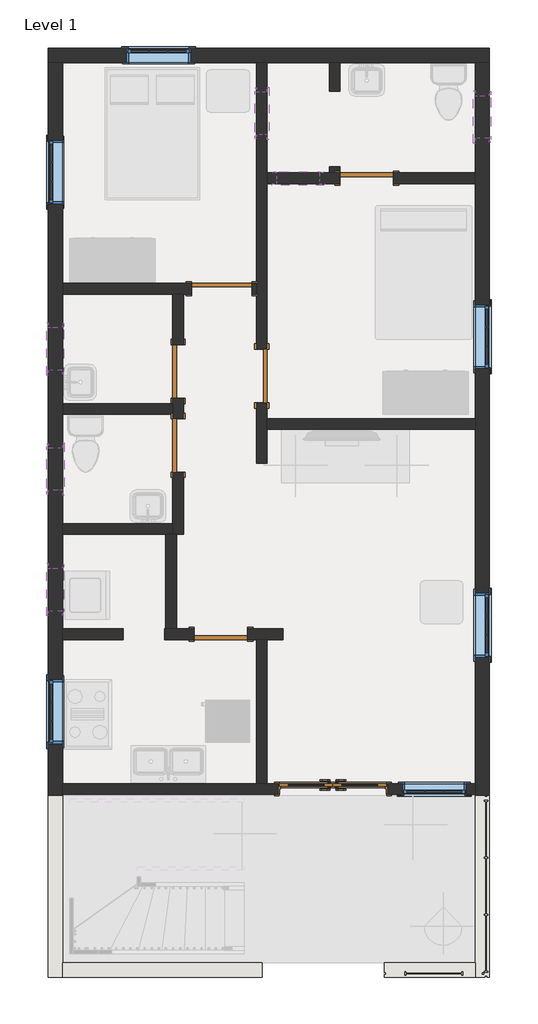
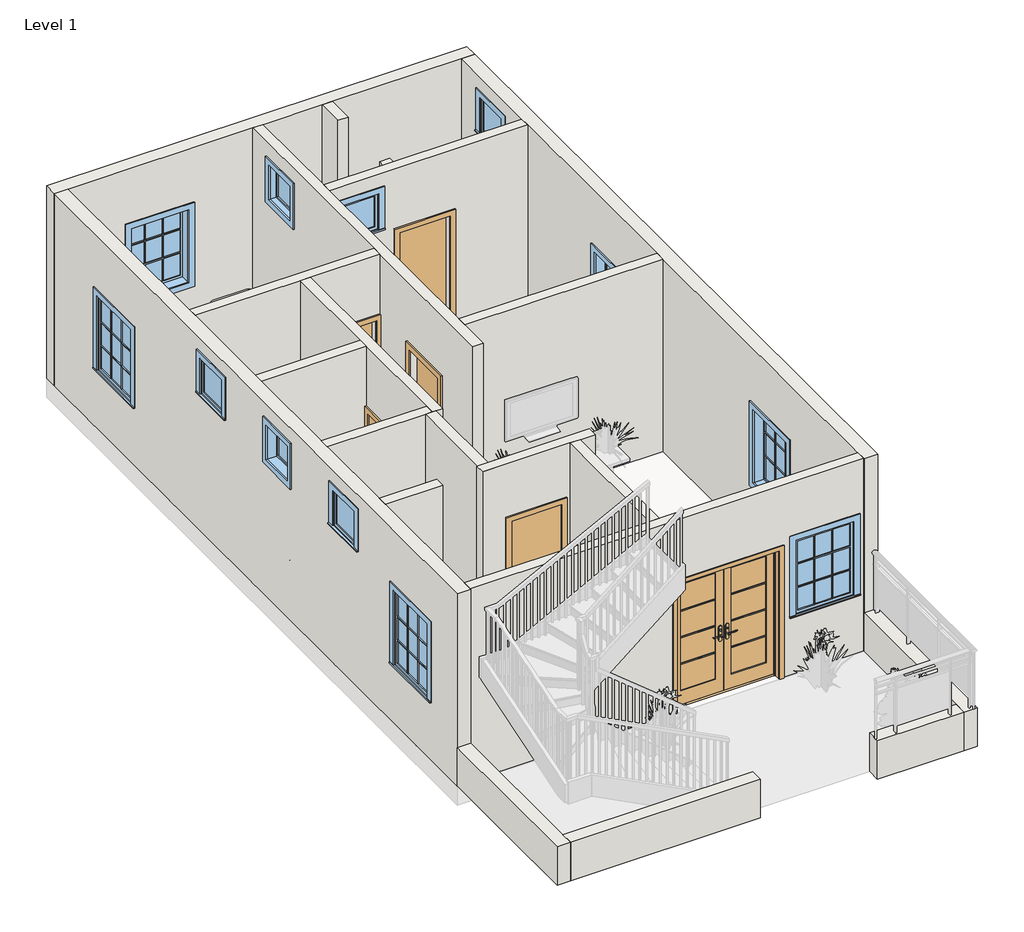
# One storey, part 1 of 3: 21 walls, 12 windows, 7 doors.
"""IFC4 building model written with IfcOpenShell, lengths in millimetres."""

from ifc_helpers import new_model, si_unit, origin, origin_with_axes, place, context, project, spatial, polyline, outline, extrude, faceted_brep, transform, mapped, element, save
from components import door_94998e6c, door_255cab33, door_059fdd7e, door_e2b13fe9, door_56e8e0a9, window_29c06734, window_5c190c7e, window_e41d21a6, window_3d781103

model = new_model("IFC4")

# Units and contexts
model_context = context("Model", 3, world=origin())
ifc_project = project(units=[si_unit("LENGTHUNIT", "METRE", prefix="MILLI")], contexts=[model_context])

# Site, building, storey
site = spatial("IfcSite", under=ifc_project)
building = spatial("IfcBuilding", under=site)
storey = spatial("IfcBuildingStorey", under=building, Name="Level 1", Elevation=0.0)

# Doors
placement = place(None, origin())
door_shape = door_94998e6c(model_context)
element("IfcDoor", 1, ObjectType="Door-Exterior-Double-Full Glass-Wood_Clad : 60\" x 80\"", at=placement, inside=storey, context=model_context, shape_type="MappedRepresentation", body=[
    mapped(door_shape, transform((-11996.3757671, 5758.0168963, 0.0), x_axis=(1.0, 0.0, 0.0), y_axis=(0.0, 1.0, 0.0), z_axis=(0.0, 0.0, 1.0))),
])
door_2_shape = door_255cab33(model_context)
element("IfcDoor", 2, ObjectType="Single-Flush : 30\" x 80\"", at=placement, inside=storey, context=model_context, shape_type="MappedRepresentation", body=[
    mapped(door_2_shape, transform((-14206.1757671, 11711.1418963, 0.0), x_axis=(0.0, -1.0, 0.0), y_axis=(1.0, 0.0, 0.0), z_axis=(0.0, 0.0, 1.0))),
])
element("IfcDoor", 3, ObjectType="Single-Flush : 30\" x 80\"", at=placement, inside=storey, context=model_context, shape_type="MappedRepresentation", body=[
    mapped(door_2_shape, transform((-11513.7757671, 14467.0418963, 0.0), x_axis=(-1.0, 0.0, 0.0), y_axis=(0.0, -1.0, 0.0), z_axis=(0.0, 0.0, 1.0))),
])
door_3_shape = door_059fdd7e(model_context)
element("IfcDoor", 4, ObjectType="Single-Flush : 30\" x 80\"", at=placement, inside=storey, context=model_context, shape_type="MappedRepresentation", body=[
    mapped(door_3_shape, transform((-14206.1757671, 10657.0418963, 0.0), x_axis=(0.0, 1.0, 0.0), y_axis=(-1.0, 0.0, 0.0), z_axis=(0.0, 0.0, 1.0))),
])
element("IfcDoor", 5, ObjectType="Single-Flush : 30\" x 80\"", at=placement, inside=storey, context=model_context, shape_type="MappedRepresentation", body=[
    mapped(door_3_shape, transform((-13012.3757671, 11647.6418963, 0.0), x_axis=(0.0, -1.0, 0.0), y_axis=(1.0, 0.0, 0.0), z_axis=(0.0, 0.0, 1.0))),
])
door_4_shape = door_e2b13fe9(model_context)
element("IfcDoor", 6, ObjectType="Single-Flush : 30\" x 84\"", at=placement, inside=storey, context=model_context, shape_type="MappedRepresentation", body=[
    mapped(door_4_shape, transform((-13596.5757671, 7964.6418963, 0.0), x_axis=(1.0, 0.0, 0.0), y_axis=(0.0, 1.0, 0.0), z_axis=(0.0, 0.0, 1.0))),
])
door_5_shape = door_56e8e0a9(model_context)
element("IfcDoor", 7, ObjectType="Single-Flush : 34\" x 80\"", at=placement, inside=storey, context=model_context, shape_type="MappedRepresentation", body=[
    mapped(door_5_shape, transform((-13583.8757671, 12892.2418963, 0.0), x_axis=(1.0, 0.0, 0.0), y_axis=(0.0, 1.0, 0.0), z_axis=(0.0, 0.0, 1.0))),
])

# Walls
element("IfcWall", 8, ObjectType="Generic - 2'", at=placement, inside=storey, context=model_context, shape_type="Brep", body=[
    faceted_brep([(-16060.3757671, 5665.9418963, 0.0), (-16060.3757671, 3075.1418963, 0.0), (-16060.3757671, 3075.1418963, 609.6), (-16060.3757671, 5665.9418963, 609.6), (-15857.1757671, 5665.9418963, 0.0), (-15857.1757671, 5665.9418963, 609.6), (-15857.1757671, 3278.3418963, 609.6), (-15857.1757671, 3075.1418963, 609.6), (-15857.1757671, 3075.1418963, 0.0), (-15857.1757671, 3278.3418963, 0.0)], [[[0, 1, 2, 3]], [[4, 5, 6, 7, 8, 9]], [[1, 0, 4, 9, 8]], [[3, 2, 7, 6, 5]], [[0, 3, 5, 4]], [[2, 1, 8, 7]]]),
])
element("IfcWall", 9, ObjectType="Generic - 2'", at=placement, inside=storey, context=model_context, shape_type="SweptSolid", body=[
    extrude(outline(polyline([(-13012.3757671, 3075.1418963), (-15857.1757671, 3075.1418963), (-15857.1757671, 3278.3418963), (-13012.3757671, 3278.3418963), (-13012.3757671, 3075.1418963)])), origin_with_axes(), (0.0, 0.0, 1.0), 609.6),
])
element("IfcWall", 10, ObjectType="Generic - 2'", at=placement, inside=storey, context=model_context, shape_type="Brep", body=[
    faceted_brep([(-9964.3757671, 5665.9418963, 0.0), (-9964.3757671, 3278.3418963, 0.0), (-9964.3757671, 3075.1418963, 0.0), (-9964.3757671, 3075.1418963, 609.6), (-9964.3757671, 3278.3418963, 609.6), (-9964.3757671, 5665.9418963, 609.6), (-9761.1757671, 5665.9418963, 0.0), (-9761.1757671, 5665.9418963, 609.6), (-9761.1757671, 3075.1418963, 609.6), (-9761.1757671, 3075.1418963, 0.0)], [[[0, 1, 2, 3, 4, 5]], [[6, 7, 8, 9]], [[2, 1, 0, 6, 9]], [[5, 4, 3, 8, 7]], [[0, 5, 7, 6]], [[3, 2, 9, 8]]]),
])
element("IfcWall", 11, ObjectType="Generic - 2'", at=placement, inside=storey, context=model_context, shape_type="SweptSolid", body=[
    extrude(outline(polyline([(-11259.7757671, 3278.3418963), (-9964.3757671, 3278.3418963), (-9964.3757671, 3075.1418963), (-11259.7757671, 3075.1418963), (-11259.7757671, 3278.3418963)])), origin_with_axes(), (0.0, 0.0, 1.0), 609.6),
])
element("IfcWall", 12, ObjectType="Generic - 8\"", at=placement, inside=storey, context=model_context, shape_type="Brep", body=[
    faceted_brep([(-16060.3757671, 16118.0418963, 0.0), (-15857.1757671, 16118.0418963, 0.0), (-13088.5757671, 16118.0418963, 0.0), (-12936.1757671, 16118.0418963, 0.0), (-12047.1757671, 16118.0418963, 0.0), (-11894.7757671, 16118.0418963, 0.0), (-9964.3757671, 16118.0418963, 0.0), (-9761.1757671, 16118.0418963, 0.0), (-9761.1757671, 16118.0418963, 3048.0), (-9964.3757671, 16118.0418963, 3048.0), (-11894.7757671, 16118.0418963, 3048.0), (-12047.1757671, 16118.0418963, 3048.0), (-12936.1757671, 16118.0418963, 3048.0), (-13088.5757671, 16118.0418963, 3048.0), (-15857.1757671, 16118.0418963, 3048.0), (-16060.3757671, 16118.0418963, 3048.0), (-14028.3757671, 16118.0418963, 2133.6), (-14028.3757671, 16118.0418963, 914.4), (-14942.7757671, 16118.0418963, 914.4), (-14942.7757671, 16118.0418963, 2133.6), (-16060.3757671, 16321.2418963, 0.0), (-16060.3757671, 16321.2418963, 3048.0), (-9761.1757671, 16321.2418963, 3048.0), (-9761.1757671, 16321.2418963, 0.0), (-14028.3757671, 16321.2418963, 2133.6), (-14942.7757671, 16321.2418963, 2133.6), (-14942.7757671, 16321.2418963, 914.4), (-14028.3757671, 16321.2418963, 914.4)], [[[0, 1, 2, 3, 4, 5, 6, 7, 8, 9, 10, 11, 12, 13, 14, 15], [16, 17, 18, 19]], [[20, 21, 22, 23], [24, 25, 26, 27]], [[7, 6, 5, 4, 3, 2, 1, 0, 20, 23]], [[8, 7, 23, 22]], [[0, 15, 21, 20]], [[17, 16, 24, 27]], [[18, 17, 27, 26]], [[19, 18, 26, 25]], [[16, 19, 25, 24]], [[15, 14, 13, 12, 11, 10, 9, 8, 22, 21]]]),
])
element("IfcWall", 13, ObjectType="Generic - 8\"", at=placement, inside=storey, context=model_context, shape_type="Brep", body=[
    faceted_brep([(-9964.3757671, 16118.0418963, 0.0), (-9964.3757671, 14543.2418963, 0.0), (-9964.3757671, 14390.8418963, 0.0), (-9964.3757671, 11038.0418963, 0.0), (-9964.3757671, 10885.6418963, 0.0), (-9964.3757671, 5831.0418963, 0.0), (-9964.3757671, 5678.6418963, 0.0), (-9964.3757671, 5665.9418963, 0.0), (-9964.3757671, 5665.9418963, 3048.0), (-9964.3757671, 5678.6418963, 3048.0), (-9964.3757671, 5831.0418963, 3048.0), (-9964.3757671, 10885.6418963, 3048.0), (-9964.3757671, 11038.0418963, 3048.0), (-9964.3757671, 14390.8418963, 3048.0), (-9964.3757671, 14543.2418963, 3048.0), (-9964.3757671, 16118.0418963, 3048.0), (-9964.3757671, 7634.4418963, 2133.6), (-9964.3757671, 7634.4418963, 914.4), (-9964.3757671, 8548.8418963, 914.4), (-9964.3757671, 8548.8418963, 2133.6), (-9964.3757671, 11749.2418963, 2133.6), (-9964.3757671, 11749.2418963, 914.4), (-9964.3757671, 12663.6418963, 914.4), (-9964.3757671, 12663.6418963, 2133.6), (-9964.3757671, 15648.1418963, 2768.6), (-9964.3757671, 15038.5418963, 2768.6), (-9964.3757671, 15038.5418963, 2159.0), (-9964.3757671, 15648.1418963, 2159.0), (-9761.1757671, 16118.0418963, 0.0), (-9761.1757671, 16118.0418963, 3048.0), (-9761.1757671, 5665.9418963, 3048.0), (-9761.1757671, 5665.9418963, 0.0), (-9761.1757671, 7634.4418963, 2133.6), (-9761.1757671, 8548.8418963, 2133.6), (-9761.1757671, 8548.8418963, 914.4), (-9761.1757671, 7634.4418963, 914.4), (-9761.1757671, 11749.2418963, 2133.6), (-9761.1757671, 12663.6418963, 2133.6), (-9761.1757671, 12663.6418963, 914.4), (-9761.1757671, 11749.2418963, 914.4), (-9761.1757671, 15648.1418963, 2768.6), (-9761.1757671, 15648.1418963, 2159.0), (-9761.1757671, 15038.5418963, 2159.0), (-9761.1757671, 15038.5418963, 2768.6)], [[[0, 1, 2, 3, 4, 5, 6, 7, 8, 9, 10, 11, 12, 13, 14, 15], [16, 17, 18, 19], [20, 21, 22, 23], [24, 25, 26, 27]], [[28, 29, 30, 31], [32, 33, 34, 35], [36, 37, 38, 39], [40, 41, 42, 43]], [[7, 6, 5, 4, 3, 2, 1, 0, 28, 31]], [[8, 7, 31, 30]], [[0, 15, 29, 28]], [[17, 16, 32, 35]], [[18, 17, 35, 34]], [[19, 18, 34, 33]], [[16, 19, 33, 32]], [[21, 20, 36, 39]], [[22, 21, 39, 38]], [[23, 22, 38, 37]], [[20, 23, 37, 36]], [[41, 40, 24, 27]], [[42, 41, 27, 26]], [[43, 42, 26, 25]], [[40, 43, 25, 24]], [[15, 14, 13, 12, 11, 10, 9, 8, 30, 29]]]),
])
element("IfcWall", 14, ObjectType="Generic - 8\"", at=placement, inside=storey, context=model_context, shape_type="Brep", body=[
    faceted_brep([(-15857.1757671, 5665.9418963, 0.0), (-15857.1757671, 5678.6418963, 0.0), (-15857.1757671, 5831.0418963, 0.0), (-15857.1757671, 7888.4418963, 0.0), (-15857.1757671, 8040.8418963, 0.0), (-15857.1757671, 9387.0418963, 0.0), (-15857.1757671, 9539.4418963, 0.0), (-15857.1757671, 11101.5418963, 0.0), (-15857.1757671, 11253.9418963, 0.0), (-15857.1757671, 12816.0418963, 0.0), (-15857.1757671, 12968.4418963, 0.0), (-15857.1757671, 16118.0418963, 0.0), (-15857.1757671, 16118.0418963, 3048.0), (-15857.1757671, 12968.4418963, 3048.0), (-15857.1757671, 12816.0418963, 3048.0), (-15857.1757671, 11253.9418963, 3048.0), (-15857.1757671, 11101.5418963, 3048.0), (-15857.1757671, 9539.4418963, 3048.0), (-15857.1757671, 9387.0418963, 3048.0), (-15857.1757671, 8040.8418963, 3048.0), (-15857.1757671, 7888.4418963, 3048.0), (-15857.1757671, 5831.0418963, 3048.0), (-15857.1757671, 5678.6418963, 3048.0), (-15857.1757671, 5665.9418963, 3048.0), (-15857.1757671, 15013.1418963, 2133.6), (-15857.1757671, 15013.1418963, 914.4), (-15857.1757671, 14098.7418963, 914.4), (-15857.1757671, 14098.7418963, 2133.6), (-15857.1757671, 7316.9418963, 2133.6), (-15857.1757671, 7316.9418963, 914.4), (-15857.1757671, 6402.5418963, 914.4), (-15857.1757671, 6402.5418963, 2133.6), (-15857.1757671, 12339.7918963, 2768.6), (-15857.1757671, 12339.7918963, 2159.0), (-15857.1757671, 11730.1918963, 2159.0), (-15857.1757671, 11730.1918963, 2768.6), (-15857.1757671, 10015.6918963, 2768.6), (-15857.1757671, 10625.2918963, 2768.6), (-15857.1757671, 10625.2918963, 2159.0), (-15857.1757671, 10015.6918963, 2159.0), (-15857.1757671, 8904.4418963, 2768.6), (-15857.1757671, 8904.4418963, 2159.0), (-15857.1757671, 8294.8418963, 2159.0), (-15857.1757671, 8294.8418963, 2768.6), (-16060.3757671, 5665.9418963, 0.0), (-16060.3757671, 5665.9418963, 3048.0), (-16060.3757671, 16118.0418963, 3048.0), (-16060.3757671, 16118.0418963, 0.0), (-16060.3757671, 15013.1418963, 2133.6), (-16060.3757671, 14098.7418963, 2133.6), (-16060.3757671, 14098.7418963, 914.4), (-16060.3757671, 15013.1418963, 914.4), (-16060.3757671, 7316.9418963, 2133.6), (-16060.3757671, 6402.5418963, 2133.6), (-16060.3757671, 6402.5418963, 914.4), (-16060.3757671, 7316.9418963, 914.4), (-16060.3757671, 12339.7918963, 2768.6), (-16060.3757671, 11730.1918963, 2768.6), (-16060.3757671, 11730.1918963, 2159.0), (-16060.3757671, 12339.7918963, 2159.0), (-16060.3757671, 10015.6918963, 2768.6), (-16060.3757671, 10015.6918963, 2159.0), (-16060.3757671, 10625.2918963, 2159.0), (-16060.3757671, 10625.2918963, 2768.6), (-16060.3757671, 8904.4418963, 2768.6), (-16060.3757671, 8294.8418963, 2768.6), (-16060.3757671, 8294.8418963, 2159.0), (-16060.3757671, 8904.4418963, 2159.0)], [[[0, 1, 2, 3, 4, 5, 6, 7, 8, 9, 10, 11, 12, 13, 14, 15, 16, 17, 18, 19, 20, 21, 22, 23], [24, 25, 26, 27], [28, 29, 30, 31], [32, 33, 34, 35], [36, 37, 38, 39], [40, 41, 42, 43]], [[44, 45, 46, 47], [48, 49, 50, 51], [52, 53, 54, 55], [56, 57, 58, 59], [60, 61, 62, 63], [64, 65, 66, 67]], [[11, 10, 9, 8, 7, 6, 5, 4, 3, 2, 1, 0, 44, 47]], [[0, 23, 45, 44]], [[12, 11, 47, 46]], [[25, 24, 48, 51]], [[26, 25, 51, 50]], [[27, 26, 50, 49]], [[24, 27, 49, 48]], [[29, 28, 52, 55]], [[30, 29, 55, 54]], [[31, 30, 54, 53]], [[28, 31, 53, 52]], [[33, 32, 56, 59]], [[34, 33, 59, 58]], [[35, 34, 58, 57]], [[32, 35, 57, 56]], [[61, 60, 36, 39]], [[62, 61, 39, 38]], [[63, 62, 38, 37]], [[60, 63, 37, 36]], [[41, 40, 64, 67]], [[42, 41, 67, 66]], [[43, 42, 66, 65]], [[40, 43, 65, 64]], [[23, 22, 21, 20, 19, 18, 17, 16, 15, 14, 13, 12, 46, 45]]]),
])
element("IfcWall", 15, ObjectType="INNER 6\"", at=placement, inside=storey, context=model_context, shape_type="Brep", body=[
    faceted_brep([(-13088.5757671, 11266.6418963, 2032.0), (-13088.5757671, 11266.6418963, 0.0), (-13088.5757671, 10403.0418963, 0.0), (-13088.5757671, 10403.0418963, 3048.0), (-13088.5757671, 12816.0418963, 3048.0), (-13088.5757671, 12968.4418963, 3048.0), (-13088.5757671, 16118.0418963, 3048.0), (-13088.5757671, 16118.0418963, 0.0), (-13088.5757671, 12968.4418963, 0.0), (-13088.5757671, 12816.0418963, 0.0), (-13088.5757671, 12028.6418963, 0.0), (-13088.5757671, 12028.6418963, 2032.0), (-13088.5757671, 15089.3418963, 2768.6), (-13088.5757671, 15089.3418963, 2159.0), (-13088.5757671, 15698.9418963, 2159.0), (-13088.5757671, 15698.9418963, 2768.6), (-12936.1757671, 10403.0418963, 0.0), (-12936.1757671, 10885.6418963, 0.0), (-12936.1757671, 11038.0418963, 0.0), (-12936.1757671, 11266.6418963, 0.0), (-12936.1757671, 11266.6418963, 2032.0), (-12936.1757671, 12028.6418963, 2032.0), (-12936.1757671, 12028.6418963, 0.0), (-12936.1757671, 14390.8418963, 0.0), (-12936.1757671, 14543.2418963, 0.0), (-12936.1757671, 16118.0418963, 0.0), (-12936.1757671, 16118.0418963, 3048.0), (-12936.1757671, 14543.2418963, 3048.0), (-12936.1757671, 14390.8418963, 3048.0), (-12936.1757671, 11038.0418963, 3048.0), (-12936.1757671, 10885.6418963, 3048.0), (-12936.1757671, 10403.0418963, 3048.0), (-12936.1757671, 15089.3418963, 2768.6), (-12936.1757671, 15698.9418963, 2768.6), (-12936.1757671, 15698.9418963, 2159.0), (-12936.1757671, 15089.3418963, 2159.0)], [[[0, 1, 2, 3, 4, 5, 6, 7, 8, 9, 10, 11], [12, 13, 14, 15]], [[16, 17, 18, 19, 20, 21, 22, 23, 24, 25, 26, 27, 28, 29, 30, 31], [32, 33, 34, 35]], [[2, 1, 19, 18, 17, 16]], [[10, 9, 8, 7, 25, 24, 23, 22]], [[3, 2, 16, 31]], [[7, 6, 26, 25]], [[20, 19, 1, 0]], [[21, 20, 0, 11]], [[22, 21, 11, 10]], [[13, 12, 32, 35]], [[14, 13, 35, 34]], [[15, 14, 34, 33]], [[12, 15, 33, 32]], [[6, 5, 4, 3, 31, 30, 29, 28, 27, 26]]]),
])
element("IfcWall", 16, ObjectType="INNER 6\"", at=placement, inside=storey, context=model_context, shape_type="Brep", body=[
    faceted_brep([(-13088.5757671, 12968.4418963, 0.0), (-13152.0757671, 12968.4418963, 0.0), (-13152.0757671, 12968.4418963, 2032.0), (-14015.6757671, 12968.4418963, 2032.0), (-14015.6757671, 12968.4418963, 0.0), (-15857.1757671, 12968.4418963, 0.0), (-15857.1757671, 12968.4418963, 3048.0), (-13088.5757671, 12968.4418963, 3048.0), (-13152.0757671, 12816.0418963, 2032.0), (-13152.0757671, 12816.0418963, 0.0), (-13088.5757671, 12816.0418963, 0.0), (-13088.5757671, 12816.0418963, 3048.0), (-14129.9757671, 12816.0418963, 3048.0), (-14282.3757671, 12816.0418963, 3048.0), (-15857.1757671, 12816.0418963, 3048.0), (-15857.1757671, 12816.0418963, 0.0), (-14282.3757671, 12816.0418963, 0.0), (-14129.9757671, 12816.0418963, 0.0), (-14015.6757671, 12816.0418963, 0.0), (-14015.6757671, 12816.0418963, 2032.0)], [[[0, 1, 2, 3, 4, 5, 6, 7]], [[8, 9, 10, 11, 12, 13, 14, 15, 16, 17, 18, 19]], [[10, 9, 1, 0]], [[18, 17, 16, 15, 5, 4]], [[0, 7, 11, 10]], [[6, 5, 15, 14]], [[2, 1, 9, 8]], [[3, 2, 8, 19]], [[4, 3, 19, 18]], [[7, 6, 14, 13, 12, 11]]]),
])
element("IfcWall", 17, ObjectType="INNER 6\"", at=placement, inside=storey, context=model_context, shape_type="SweptSolid", body=[
    extrude(outline(polyline([(-9964.3757671, 10885.6418963), (-12936.1757671, 10885.6418963), (-12936.1757671, 11038.0418963), (-9964.3757671, 11038.0418963), (-9964.3757671, 10885.6418963)])), origin_with_axes(), (0.0, 0.0, 1.0), 3048.0),
])
element("IfcWall", 18, ObjectType="INNER 6\"", at=placement, inside=storey, context=model_context, shape_type="Brep", body=[
    faceted_brep([(-14282.3757671, 11330.1418963, 2032.0), (-14282.3757671, 11330.1418963, 0.0), (-14282.3757671, 11253.9418963, 0.0), (-14282.3757671, 11101.5418963, 0.0), (-14282.3757671, 11038.0418963, 0.0), (-14282.3757671, 11038.0418963, 2032.0), (-14282.3757671, 10276.0418963, 2032.0), (-14282.3757671, 10276.0418963, 0.0), (-14282.3757671, 9539.4418963, 0.0), (-14282.3757671, 9387.0418963, 0.0), (-14282.3757671, 9387.0418963, 3048.0), (-14282.3757671, 9539.4418963, 3048.0), (-14282.3757671, 11101.5418963, 3048.0), (-14282.3757671, 11253.9418963, 3048.0), (-14282.3757671, 12816.0418963, 3048.0), (-14282.3757671, 12816.0418963, 0.0), (-14282.3757671, 12092.1418963, 0.0), (-14282.3757671, 12092.1418963, 2032.0), (-14129.9757671, 11038.0418963, 0.0), (-14129.9757671, 11330.1418963, 0.0), (-14129.9757671, 11330.1418963, 2032.0), (-14129.9757671, 12092.1418963, 2032.0), (-14129.9757671, 12092.1418963, 0.0), (-14129.9757671, 12816.0418963, 0.0), (-14129.9757671, 12816.0418963, 3048.0), (-14129.9757671, 9387.0418963, 3048.0), (-14129.9757671, 9387.0418963, 0.0), (-14129.9757671, 10276.0418963, 0.0), (-14129.9757671, 10276.0418963, 2032.0), (-14129.9757671, 11038.0418963, 2032.0), (-14231.5757671, 9387.0418963, 0.0), (-14231.5757671, 9387.0418963, 3048.0)], [[[0, 1, 2, 3, 4, 5, 6, 7, 8, 9, 10, 11, 12, 13, 14, 15, 16, 17]], [[18, 19, 20, 21, 22, 23, 24, 25, 26, 27, 28, 29]], [[27, 26, 30, 9, 8, 7]], [[16, 15, 23, 22]], [[4, 3, 2, 1, 19, 18]], [[15, 14, 24, 23]], [[10, 9, 30, 26, 25, 31]], [[5, 4, 18, 29]], [[6, 5, 29, 28]], [[7, 6, 28, 27]], [[20, 19, 1, 0]], [[21, 20, 0, 17]], [[22, 21, 17, 16]], [[14, 13, 12, 11, 10, 31, 25, 24]]]),
])
element("IfcWall", 19, ObjectType="INNER 6\"", at=placement, inside=storey, context=model_context, shape_type="Brep", body=[
    faceted_brep([(-14282.3757671, 9539.4418963, 0.0), (-15857.1757671, 9539.4418963, 0.0), (-15857.1757671, 9539.4418963, 3048.0), (-14282.3757671, 9539.4418963, 3048.0), (-14282.3757671, 9387.0418963, 0.0), (-14282.3757671, 9387.0418963, 3048.0), (-14383.9757671, 9387.0418963, 3048.0), (-15857.1757671, 9387.0418963, 3048.0), (-15857.1757671, 9387.0418963, 0.0), (-14383.9757671, 9387.0418963, 0.0)], [[[0, 1, 2, 3]], [[4, 5, 6, 7, 8, 9]], [[1, 0, 4, 9, 8]], [[0, 3, 5, 4]], [[2, 1, 8, 7]], [[3, 2, 7, 6, 5]]]),
])
element("IfcWall", 20, ObjectType="INNER 6\"", at=placement, inside=storey, context=model_context, shape_type="Brep", body=[
    faceted_brep([(-14383.9757671, 9387.0418963, 0.0), (-14383.9757671, 7888.4418963, 0.0), (-14383.9757671, 7888.4418963, 3048.0), (-14383.9757671, 9387.0418963, 3048.0), (-14231.5757671, 9387.0418963, 0.0), (-14231.5757671, 9387.0418963, 3048.0), (-14231.5757671, 7888.4418963, 3048.0), (-14231.5757671, 7888.4418963, 0.0), (-14282.3757671, 9387.0418963, 0.0), (-14282.3757671, 9387.0418963, 3048.0)], [[[0, 1, 2, 3]], [[4, 5, 6, 7]], [[1, 0, 8, 4, 7]], [[2, 1, 7, 6]], [[0, 3, 9, 5, 4, 8]], [[3, 2, 6, 5, 9]]]),
])
element("IfcWall", 21, ObjectType="INNER 6\"", at=placement, inside=storey, context=model_context, shape_type="Brep", body=[
    faceted_brep([(-12707.5757671, 8040.8418963, 0.0), (-13215.5757671, 8040.8418963, 0.0), (-13215.5757671, 8040.8418963, 2133.6), (-13977.5757671, 8040.8418963, 2133.6), (-13977.5757671, 8040.8418963, 0.0), (-14396.6757671, 8040.8418963, 0.0), (-14396.6757671, 8040.8418963, 3048.0), (-12707.5757671, 8040.8418963, 3048.0), (-13215.5757671, 7888.4418963, 2133.6), (-13215.5757671, 7888.4418963, 0.0), (-13088.5757671, 7888.4418963, 0.0), (-12936.1757671, 7888.4418963, 0.0), (-12707.5757671, 7888.4418963, 0.0), (-12707.5757671, 7888.4418963, 3048.0), (-12936.1757671, 7888.4418963, 3048.0), (-13088.5757671, 7888.4418963, 3048.0), (-14396.6757671, 7888.4418963, 3048.0), (-14396.6757671, 7888.4418963, 0.0), (-13977.5757671, 7888.4418963, 0.0), (-13977.5757671, 7888.4418963, 2133.6)], [[[0, 1, 2, 3, 4, 5, 6, 7]], [[8, 9, 10, 11, 12, 13, 14, 15, 16, 17, 18, 19]], [[18, 17, 5, 4]], [[12, 11, 10, 9, 1, 0]], [[6, 5, 17, 16]], [[0, 7, 13, 12]], [[2, 1, 9, 8]], [[3, 2, 8, 19]], [[4, 3, 19, 18]], [[7, 6, 16, 15, 14, 13]]]),
])
element("IfcWall", 22, ObjectType="INNER 6\"", at=placement, inside=storey, context=model_context, shape_type="SweptSolid", body=[
    extrude(outline(polyline([(-13088.5757671, 5831.0418963), (-13088.5757671, 7888.4418963), (-12936.1757671, 7888.4418963), (-12936.1757671, 5831.0418963), (-13088.5757671, 5831.0418963)])), origin_with_axes(), (0.0, 0.0, 1.0), 3048.0),
])
element("IfcWall", 23, ObjectType="INNER 6\"", at=placement, inside=storey, context=model_context, shape_type="Brep", body=[
    faceted_brep([(-15857.1757671, 5831.0418963, 0.0), (-15857.1757671, 5831.0418963, 3048.0), (-13088.5757671, 5831.0418963, 3048.0), (-12936.1757671, 5831.0418963, 3048.0), (-9964.3757671, 5831.0418963, 3048.0), (-9964.3757671, 5831.0418963, 0.0), (-11208.9757671, 5831.0418963, 0.0), (-11208.9757671, 5831.0418963, 2057.4), (-12783.7757671, 5831.0418963, 2057.4), (-12783.7757671, 5831.0418963, 0.0), (-12936.1757671, 5831.0418963, 0.0), (-13088.5757671, 5831.0418963, 0.0), (-11005.7757671, 5831.0418963, 2133.6), (-11005.7757671, 5831.0418963, 914.4), (-10091.3757671, 5831.0418963, 914.4), (-10091.3757671, 5831.0418963, 2133.6), (-15857.1757671, 5678.6418963, 3048.0), (-15857.1757671, 5678.6418963, 0.0), (-12783.7757671, 5678.6418963, 0.0), (-12783.7757671, 5678.6418963, 2057.4), (-11208.9757671, 5678.6418963, 2057.4), (-11208.9757671, 5678.6418963, 0.0), (-9964.3757671, 5678.6418963, 0.0), (-9964.3757671, 5678.6418963, 3048.0), (-11005.7757671, 5678.6418963, 2133.6), (-10091.3757671, 5678.6418963, 2133.6), (-10091.3757671, 5678.6418963, 914.4), (-11005.7757671, 5678.6418963, 914.4)], [[[0, 1, 2, 3, 4, 5, 6, 7, 8, 9, 10, 11], [12, 13, 14, 15]], [[16, 17, 18, 19, 20, 21, 22, 23], [24, 25, 26, 27]], [[17, 0, 11, 10, 9, 18]], [[5, 22, 21, 6]], [[1, 0, 17, 16]], [[20, 7, 6, 21]], [[7, 20, 19, 8]], [[8, 19, 18, 9]], [[13, 12, 24, 27]], [[14, 13, 27, 26]], [[15, 14, 26, 25]], [[12, 15, 25, 24]], [[5, 4, 23, 22]], [[4, 3, 2, 1, 16, 23]]]),
])
element("IfcWall", 24, ObjectType="INNER 6\"", at=placement, inside=storey, context=model_context, shape_type="SweptSolid", body=[
    extrude(outline(polyline([(-15857.1757671, 11253.9418963), (-14282.3757671, 11253.9418963), (-14282.3757671, 11101.5418963), (-15857.1757671, 11101.5418963), (-15857.1757671, 11253.9418963)])), origin_with_axes(), (0.0, 0.0, 1.0), 3048.0),
])
element("IfcWall", 25, ObjectType="INNER 6\"", at=placement, inside=storey, context=model_context, shape_type="Brep", body=[
    faceted_brep([(-12936.1757671, 14390.8418963, 0.0), (-11894.7757671, 14390.8418963, 0.0), (-11894.7757671, 14390.8418963, 2032.0), (-11132.7757671, 14390.8418963, 2032.0), (-11132.7757671, 14390.8418963, 0.0), (-9964.3757671, 14390.8418963, 0.0), (-9964.3757671, 14390.8418963, 3048.0), (-12936.1757671, 14390.8418963, 3048.0), (-12796.4757671, 14390.8418963, 2768.6), (-12186.8757671, 14390.8418963, 2768.6), (-12186.8757671, 14390.8418963, 2159.0), (-12796.4757671, 14390.8418963, 2159.0), (-11894.7757671, 14543.2418963, 2032.0), (-11894.7757671, 14543.2418963, 0.0), (-12047.1757671, 14543.2418963, 0.0), (-12936.1757671, 14543.2418963, 0.0), (-12936.1757671, 14543.2418963, 3048.0), (-12047.1757671, 14543.2418963, 3048.0), (-11894.7757671, 14543.2418963, 3048.0), (-9964.3757671, 14543.2418963, 3048.0), (-9964.3757671, 14543.2418963, 0.0), (-11132.7757671, 14543.2418963, 0.0), (-11132.7757671, 14543.2418963, 2032.0), (-12796.4757671, 14543.2418963, 2768.6), (-12796.4757671, 14543.2418963, 2159.0), (-12186.8757671, 14543.2418963, 2159.0), (-12186.8757671, 14543.2418963, 2768.6)], [[[0, 1, 2, 3, 4, 5, 6, 7], [8, 9, 10, 11]], [[12, 13, 14, 15, 16, 17, 18, 19, 20, 21, 22], [23, 24, 25, 26]], [[21, 20, 5, 4]], [[15, 14, 13, 1, 0]], [[6, 5, 20, 19]], [[0, 7, 16, 15]], [[2, 1, 13, 12]], [[3, 2, 12, 22]], [[4, 3, 22, 21]], [[24, 23, 8, 11]], [[25, 24, 11, 10]], [[26, 25, 10, 9]], [[23, 26, 9, 8]], [[7, 6, 19, 18, 17, 16]]]),
])
element("IfcWall", 26, ObjectType="INNER 6\"", at=placement, inside=storey, context=model_context, shape_type="Brep", body=[
    faceted_brep([(-12047.1757671, 14632.1418963, 0.0), (-12047.1757671, 14543.2418963, 0.0), (-12047.1757671, 14543.2418963, 3048.0), (-12047.1757671, 14632.1418963, 3048.0), (-11894.7757671, 14632.1418963, 0.0), (-11894.7757671, 14632.1418963, 3048.0), (-11894.7757671, 14543.2418963, 3048.0), (-11894.7757671, 14543.2418963, 2032.0), (-11894.7757671, 14543.2418963, 0.0)], [[[0, 1, 2, 3]], [[4, 5, 6, 7, 8]], [[1, 0, 4, 8]], [[0, 3, 5, 4]], [[2, 1, 8, 7, 6]], [[3, 2, 6, 5]]]),
])
element("IfcWall", 27, ObjectType="INNER 6\"", at=placement, inside=storey, context=model_context, shape_type="SweptSolid", body=[
    extrude(outline(polyline([(-12047.1757671, 15711.6418963), (-12047.1757671, 16118.0418963), (-11894.7757671, 16118.0418963), (-11894.7757671, 15711.6418963), (-12047.1757671, 15711.6418963)])), origin_with_axes(), (0.0, 0.0, 1.0), 3048.0),
])
element("IfcWall", 28, ObjectType="INNER 6\"", at=placement, inside=storey, context=model_context, shape_type="SweptSolid", body=[
    extrude(outline(polyline([(-15857.1757671, 8040.8418963), (-14993.5757671, 8040.8418963), (-14993.5757671, 7888.4418963), (-15857.1757671, 7888.4418963), (-15857.1757671, 8040.8418963)])), origin_with_axes(), (0.0, 0.0, 1.0), 3048.0),
])

# Windows
window_shape = window_29c06734(model_context)
element("IfcWindow", 29, ObjectType="Casement 3x3 with Trim : 36\" x 48\"", at=placement, inside=storey, context=model_context, shape_type="MappedRepresentation", body=[
    mapped(window_shape, transform((-14485.5757671, 16219.6418963, 0.0), x_axis=(1.0, 0.0, 0.0), y_axis=(0.0, 1.0, 0.0), z_axis=(0.0, 0.0, 1.0))),
])
element("IfcWindow", 30, ObjectType="Casement 3x3 with Trim : 36\" x 48\"", at=placement, inside=storey, context=model_context, shape_type="MappedRepresentation", body=[
    mapped(window_shape, transform((-15958.7757671, 14555.9418963, 0.0), x_axis=(0.0, 1.0, 0.0), y_axis=(-1.0, 0.0, 0.0), z_axis=(0.0, 0.0, 1.0))),
])
element("IfcWindow", 31, ObjectType="Casement 3x3 with Trim : 36\" x 48\"", at=placement, inside=storey, context=model_context, shape_type="MappedRepresentation", body=[
    mapped(window_shape, transform((-15958.7757671, 6859.7418963, 0.0), x_axis=(0.0, 1.0, 0.0), y_axis=(-1.0, 0.0, 0.0), z_axis=(0.0, 0.0, 1.0))),
])
element("IfcWindow", 32, ObjectType="Casement 3x3 with Trim : 36\" x 48\"", at=placement, inside=storey, context=model_context, shape_type="MappedRepresentation", body=[
    mapped(window_shape, transform((-9862.7757671, 8091.6418963, 0.0), x_axis=(0.0, -1.0, 0.0), y_axis=(1.0, 0.0, 0.0), z_axis=(0.0, 0.0, 1.0))),
])
element("IfcWindow", 33, ObjectType="Casement 3x3 with Trim : 36\" x 48\"", at=placement, inside=storey, context=model_context, shape_type="MappedRepresentation", body=[
    mapped(window_shape, transform((-9862.7757671, 12206.4418963, 0.0), x_axis=(0.0, -1.0, 0.0), y_axis=(1.0, 0.0, 0.0), z_axis=(0.0, 0.0, 1.0))),
])
window_2_shape = window_5c190c7e(model_context)
element("IfcWindow", 34, ObjectType="Casement 3x3 with Trim : 36\" x 48\"", at=placement, inside=storey, context=model_context, shape_type="MappedRepresentation", body=[
    mapped(window_2_shape, transform((-10548.5757671, 5754.8418963, 0.0), x_axis=(-1.0, 0.0, 0.0), y_axis=(0.0, -1.0, 0.0), z_axis=(0.0, 0.0, 1.0))),
])
window_3_shape = window_e41d21a6(model_context)
element("IfcWindow", 35, ObjectType="Transom with Trim : 24\" x 24\"", at=placement, inside=storey, context=model_context, shape_type="MappedRepresentation", body=[
    mapped(window_3_shape, transform((-9862.7757671, 15381.4418963, 0.0), x_axis=(0.0, 1.0, 0.0), y_axis=(-1.0, 0.0, 0.0), z_axis=(0.0, 0.0, 1.0))),
])
element("IfcWindow", 36, ObjectType="Transom with Trim : 24\" x 24\"", at=placement, inside=storey, context=model_context, shape_type="MappedRepresentation", body=[
    mapped(window_3_shape, transform((-15958.7757671, 12073.0918963, 0.0), x_axis=(0.0, 1.0, 0.0), y_axis=(-1.0, 0.0, 0.0), z_axis=(0.0, 0.0, 1.0))),
])
element("IfcWindow", 37, ObjectType="Transom with Trim : 24\" x 24\"", at=placement, inside=storey, context=model_context, shape_type="MappedRepresentation", body=[
    mapped(window_3_shape, transform((-15958.7757671, 10282.3918963, 0.0), x_axis=(0.0, -1.0, 0.0), y_axis=(1.0, 0.0, 0.0), z_axis=(0.0, 0.0, 1.0))),
])
element("IfcWindow", 38, ObjectType="Transom with Trim : 24\" x 24\"", at=placement, inside=storey, context=model_context, shape_type="MappedRepresentation", body=[
    mapped(window_3_shape, transform((-15958.7757671, 8637.7418963, 0.0), x_axis=(0.0, 1.0, 0.0), y_axis=(-1.0, 0.0, 0.0), z_axis=(0.0, 0.0, 1.0))),
])
window_4_shape = window_3d781103(model_context)
element("IfcWindow", 39, ObjectType="Transom with Trim : 24\" x 24\"", at=placement, inside=storey, context=model_context, shape_type="MappedRepresentation", body=[
    mapped(window_4_shape, transform((-12529.7757671, 14467.0418963, 0.0), x_axis=(-1.0, 0.0, 0.0), y_axis=(0.0, -1.0, 0.0), z_axis=(0.0, 0.0, 1.0))),
])
element("IfcWindow", 40, ObjectType="Transom with Trim : 24\" x 24\"", at=placement, inside=storey, context=model_context, shape_type="MappedRepresentation", body=[
    mapped(window_4_shape, transform((-13012.3757671, 15356.0418963, 0.0), x_axis=(0.0, -1.0, 0.0), y_axis=(1.0, 0.0, 0.0), z_axis=(0.0, 0.0, 1.0))),
])

save(model, "model.ifc")

# Revit data of these elements
# Type "Door-Exterior-Double-Full Glass-Wood_Clad : 60\" x 80\""
#   Type Mark = "8"
#   Assembly Code = "B2030100"
#   Analytic Construction = "French door, wood frame with double glass"
#   Top Rail = 0' - 4 11/16"
#   Threshold Offset [instance default] = 0' - 0 1/2"
#   Thickness = 0' - 1 3/8"
#   Thermal Resistance (R) = 1.9158 (h·ft²·°F)/BTU
#   Swing Angle [instance default] = 90.00°
#   Stiles = 0' - 4 3/4"
#   Rough Width = 5' - 2"
#   Rough Height = 6' - 9"
#   Panel Width = 2' - 6"
#   Door Offset [instance default] = 0' - 0"
#   Height = 6' - 8"
#   Width = 5' - 0"
#   Heat Transfer Coefficient (U) = 0.5220 BTU/(h·ft²·°F)
#   Bottom Rail = 0' - 9 1/8"
#   Exterior Trim [instance default] = yes
#   Threshold [instance default] = yes
#   Show Grill [instance default] = yes
#   Function = 1
#   Trim Material = Cherry
#   Threshold Material = Cherry
#   Panel Material = Cherry
#   Glazing = Glass
#   Frame Material = Cherry
#   Door Handle Material = Aluminum
#   Visual Light Transmittance = 0
#   Solar Heat Gain Coefficient = 0
#   Wall Closure = (empty or 0)
#   Construction Type = (empty or 0)
# Type "Single-Flush : 30\" x 80\""
#   Type Mark = "5"
#   Construction Type Id = "MDOOR"
#   Assembly Code = "C1020"
#   Analytic Construction = "Metal"
#   Thickness = 0' - 2"
#   Heat Transfer Coefficient (U) = 0.651978 BTU/(h·ft²·°F)
#   Height = 6' - 8"
#   Trim Projection Ext = 0' - 1"
#   Trim Projection Int = 0' - 1"
#   Trim Width = 0' - 3"
#   Width = 2' - 6"
#   Define Thermal Properties by = 1
#   Door Material = Door - Panel
#   Frame Material = Door - Frame
#   Visual Light Transmittance = 0
#   Solar Heat Gain Coefficient = 0
#   Function = (empty or 0)
#   Wall Closure = (empty or 0)
# Type "Single-Flush : 30\" x 84\""
#   Type Mark = "4"
#   Construction Type Id = "MDOOR"
#   Assembly Code = "C1020"
#   Analytic Construction = "Metal"
#   Thickness = 0' - 2"
#   Heat Transfer Coefficient (U) = 0.651978 BTU/(h·ft²·°F)
#   Height = 7' - 0"
#   Trim Projection Ext = 0' - 1"
#   Trim Projection Int = 0' - 1"
#   Trim Width = 0' - 3"
#   Width = 2' - 6"
#   Define Thermal Properties by = 1
#   Door Material = Door - Panel
#   Frame Material = Door - Frame
#   Visual Light Transmittance = 0
#   Solar Heat Gain Coefficient = 0
#   Function = (empty or 0)
#   Wall Closure = (empty or 0)
# Type "Single-Flush : 34\" x 80\""
#   Type Mark = "7"
#   Construction Type Id = "MDOOR"
#   Assembly Code = "C1020"
#   Analytic Construction = "Metal"
#   Thickness = 0' - 2"
#   Heat Transfer Coefficient (U) = 0.651978 BTU/(h·ft²·°F)
#   Height = 6' - 8"
#   Trim Projection Ext = 0' - 1"
#   Trim Projection Int = 0' - 1"
#   Trim Width = 0' - 3"
#   Width = 2' - 10"
#   Define Thermal Properties by = 1
#   Door Material = Door - Panel
#   Frame Material = Door - Frame
#   Visual Light Transmittance = 0
#   Solar Heat Gain Coefficient = 0
#   Function = (empty or 0)
#   Wall Closure = (empty or 0)
# Type "Generic - 2'"
#   Assembly Code = "B2010"
#   Layers, outside or top first: 0' - 8" "Birch" (function 1)
# Type "Generic - 8\""
#   Assembly Code = "B2010"
#   Layers, outside or top first: 0' - 8" "Brick, Common" (function 1)
# Type "INNER 6\""
#   Assembly Code = "B2010"
#   Layers, outside or top first: 0' - 6" "Brick, Common" (function 1)
# Type "Casement 3x3 with Trim : 36\" x 48\""
#   Type Mark = "10"
#   Construction Type Id = "GSP4R"
#   Assembly Code = "B2020100"
#   Analytic Construction = "1/8 in Pilkington single glazing"
#   Visual Light Transmittance = 0.9
#   Solar Heat Gain Coefficient = 0.78
#   Heat Transfer Coefficient (U) = 0.6496 BTU/(h·ft²·°F)
#   Height = 4' - 0"
#   Default Sill Height = 3' - 0"
#   Trim Projection - Ext. = 0' - 0 1/2"
#   Trim Projection - Int. = 0' - 0 3/4"
#   Trim Width - Exterior = 0' - 3 1/2"
#   Trim Width - Interior = 0' - 3 1/2"
#   Width = 3' - 0"
#   Window Inset = 0' - 0 3/4"
#   Define Thermal Properties by = 1
#   Glass Pane Material = Glass
#   Sash Material = Sash
#   Trim Exterior Material = Trim
#   Trim Interior Material = Trim
#   Wall Closure = (empty or 0)
# Type "Transom with Trim : 24\" x 24\""
#   Type Mark = "13"
#   Construction Type Id = "GSP4R"
#   Assembly Code = "B2020100"
#   Analytic Construction = "1/8 in Pilkington single glazing"
#   Visual Light Transmittance = 0.9
#   Solar Heat Gain Coefficient = 0.78
#   Heat Transfer Coefficient (U) = 0.6496 BTU/(h·ft²·°F)
#   Height = 2' - 0"
#   Default Sill Height = 7' - 1"
#   Trim Projection - Ext. = 0' - 0 1/2"
#   Trim Projection - Int. = 0' - 0 3/4"
#   Trim Width - Exterior = 0' - 3 1/2"
#   Trim Width - Interior = 0' - 3 1/2"
#   Width = 2' - 0"
#   Window Inset = 0' - 0 3/4"
#   Define Thermal Properties by = 1
#   Glass Pane Material = Glass
#   Sash Material = Sash
#   Trim Exterior Material = Trim
#   Trim Interior Material = Trim
#   Wall Closure = (empty or 0)
# Element 1 (IfcDoor, "Door-Exterior-Double-Full Glass-Wood_Clad : 60\" x 80\"")
#   Threshold Offset = 0' - 0 1/2"
#   Swing Angle = 90.00°
#   Door Offset = 0' - 0"
#   Threshold = yes
#   Show Grill = yes
#   Exterior Trim = yes
#   Phase Created = New Construction
#   Materials on its faces: "Cherry", "Aluminum", "Glass"
# Elements 2, 3, 4, 5 (IfcDoor, "Single-Flush : 30\" x 80\"")
#   Phase Created = New Construction
#   Materials on its faces: "Door - Frame", "Door - Panel"
# Element 6 (IfcDoor, "Single-Flush : 30\" x 84\"")
#   Phase Created = New Construction
#   Materials on its faces: "Door - Frame", "Door - Panel"
# Element 7 (IfcDoor, "Single-Flush : 34\" x 80\"")
#   Phase Created = New Construction
#   Materials on its faces: "Door - Frame", "Door - Panel"
# Elements 8, 9, 10, 11 (IfcWall, "Generic - 2'")
#   Top Offset = 0' - 0"
#   Base Offset = 0' - 0"
#   Unconnected Height = 2' - 0"
#   wall height = 2' - 0"
#   Phase Created = New Construction
#   Base Constraint = Level 1
#   Materials on its faces: "Birch"
# Elements 12, 13, 14 (IfcWall, "Generic - 8\"")
#   Top Offset = 0' - 0"
#   Base Offset = 0' - 0"
#   Unconnected Height = 10' - 0"
#   wall height = 10' - 0"
#   Phase Created = New Construction
#   Base Constraint = Level 1
#   Materials on its faces: "Brick, Common"
# Elements 15, 16, 17, 18, 19, 20, 21, 22, 23, 24, 25, 26, 27, 28 (IfcWall, "INNER 6\"")
#   Top Offset = 0' - 0"
#   Base Offset = 0' - 0"
#   Unconnected Height = 10' - 0"
#   wall height = 10' - 0"
#   Phase Created = New Construction
#   Base Constraint = Level 1
#   Materials on its faces: "Brick, Common"
# Element 29 (IfcWindow, "Casement 3x3 with Trim : 36\" x 48\"")
#   Mark = "1"
#   Phase Created = New Construction
#   Materials on its faces: "Sash", "Glass", "Trim"
# Element 30 (IfcWindow, "Casement 3x3 with Trim : 36\" x 48\"")
#   Mark = "2"
#   Phase Created = New Construction
#   Materials on its faces: "Sash", "Glass", "Trim"
# Element 31 (IfcWindow, "Casement 3x3 with Trim : 36\" x 48\"")
#   Mark = "3"
#   Phase Created = New Construction
#   Materials on its faces: "Sash", "Glass", "Trim"
# Element 32 (IfcWindow, "Casement 3x3 with Trim : 36\" x 48\"")
#   Mark = "4"
#   Phase Created = New Construction
#   Materials on its faces: "Sash", "Glass", "Trim"
# Element 33 (IfcWindow, "Casement 3x3 with Trim : 36\" x 48\"")
#   Mark = "5"
#   Phase Created = New Construction
#   Materials on its faces: "Sash", "Glass", "Trim"
# Element 34 (IfcWindow, "Casement 3x3 with Trim : 36\" x 48\"")
#   Mark = "13"
#   Phase Created = New Construction
#   Materials on its faces: "Sash", "Glass", "Trim"
# Element 35 (IfcWindow, "Transom with Trim : 24\" x 24\"")
#   Mark = "6"
#   Phase Created = New Construction
#   Materials on its faces: "Sash", "Trim", "Glass"
# Element 36 (IfcWindow, "Transom with Trim : 24\" x 24\"")
#   Mark = "9"
#   Phase Created = New Construction
#   Materials on its faces: "Sash", "Trim", "Glass"
# Element 37 (IfcWindow, "Transom with Trim : 24\" x 24\"")
#   Mark = "10"
#   Phase Created = New Construction
#   Materials on its faces: "Sash", "Trim", "Glass"
# Element 38 (IfcWindow, "Transom with Trim : 24\" x 24\"")
#   Mark = "11"
#   Phase Created = New Construction
#   Materials on its faces: "Sash", "Trim", "Glass"
# Element 39 (IfcWindow, "Transom with Trim : 24\" x 24\"")
#   Mark = "7"
#   Phase Created = New Construction
#   Materials on its faces: "Sash", "Trim", "Glass"
# Element 40 (IfcWindow, "Transom with Trim : 24\" x 24\"")
#   Mark = "8"
#   Phase Created = New Construction
#   Materials on its faces: "Sash", "Trim", "Glass"
# Materials
#   "Cherry": class "Wood", colour RGB 226 177 128, transparency 0, Description = "Prunus Serotina", Cost = 0
#   "Glass": class "Glass", colour RGB 0 128 192, transparency 0.75, Description = "Soda Lime Glass", Cost = 0
#   "Aluminum": class "Metal", colour RGB 247 247 247, transparency 0, Description = "Aluminum 6061", Cost = 0
#   "Door - Panel": class "Wood", colour RGB 210 159 95, transparency 0
#   "Door - Frame": colour RGB 118 70 51, transparency 0
#   "Birch": class "Wood", colour RGB 224 178 126, transparency 0, Description = "Betula Alleghaniensis", Cost = 0
#   "Brick, Common": class "Masonry", colour RGB 170 98 104, transparency 0, Description = "Common brick", Cost = 0
#   "Sash": class "Wood", colour RGB 224 178 126, transparency 0
#   "Trim": class "Wood", colour RGB 224 178 126, transparency 0
# Room at (-15088.165, 11938.999) mm, phase "New Construction", upper level "Level 1", upper offset 10' - 0", lower offset 0' - 0"
#   Number = "5"
#   Name = "BATH"
# Room at (-15088.165, 10007.402) mm, phase "New Construction", upper level "Level 1", upper offset 10' - 0", lower offset 0' - 0"
#   Number = "6"
#   Name = "TOILET"
# Room at (-15088.165, 8543.707) mm, phase "New Construction", upper level "Level 1", upper offset 10' - 0", lower offset 0' - 0"
#   Number = "7"
#   Name = "WASH"
# Room at (-11604.14, 8306.077) mm, phase "New Construction", upper level "Level 1", upper offset 10' - 0", lower offset 0' - 0"
#   Number = "9"
#   Name = "HALL"
# Room at (-13610.761, 10532.174) mm, phase "New Construction", upper level "Level 1", upper offset 10' - 0", lower offset 0' - 0"
#   Number = "10"
#   Name = "PASSAGE"
# Room at (-14593.797, 14545.162) mm, phase "New Construction", upper level "Level 1", upper offset 10' - 0", lower offset 0' - 0"
#   Number = "1"
#   Name = "BEDROOM"
# Room at (-12374.351, 15136.739) mm, phase "New Construction", upper level "Level 1", upper offset 10' - 0", lower offset 0' - 0"
#   Number = "2"
# Room at (-10953.247, 15136.739) mm, phase "New Construction", upper level "Level 1", upper offset 10' - 0", lower offset 0' - 0"
#   Number = "3"
# Room at (-11604.14, 4346.984) mm, phase "New Construction", upper level "Level 1", upper offset 10' - 0", lower offset 0' - 0"
#   Number = "11"
#   Name = "PORCH"
# Room at (-14230.089, 6685.048) mm, phase "New Construction", upper level "Level 1", upper offset 10' - 0", lower offset 0' - 0"
#   Number = "8"
#   Name = "KITCHEN"
# Room at (-11442.496, 12495.328) mm, phase "New Construction", upper level "Level 1", upper offset 10' - 0", lower offset 0' - 0"
#   Number = "4"
#   Name = "BEDROOM"
